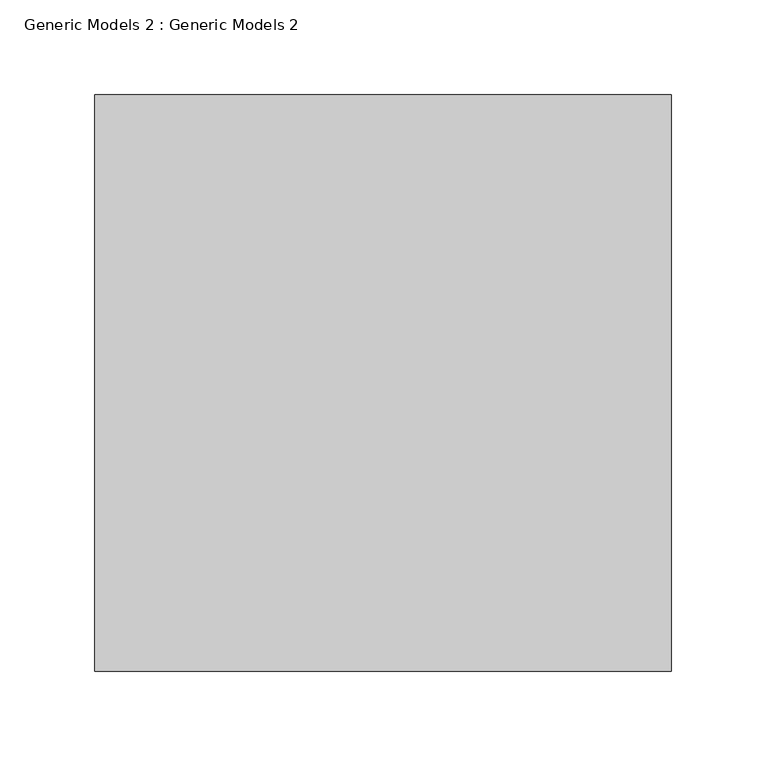
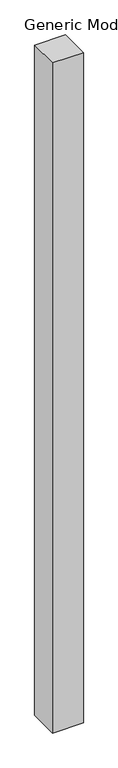
"""IFC4 building model written with IfcOpenShell, lengths in millimetres: proxy geometry, Generic Models 2 : Generic Models 2."""

from ifc_helpers import new_model, si_unit, origin, origin_with_axes, place, context, project, spatial, polyline, outline, extrude, source, transform, mapped, element, save


def generic_models_2_generic_models_2_628e6232(model_context):
    return source(origin(), model_context, "Body", "SweptSolid", [
        extrude(outline(polyline([(-8177.3519453, 3667.2444012), (-8482.1519453, 3667.2444012), (-8482.1519453, 3972.0444012), (-8177.3519453, 3972.0444012), (-8177.3519453, 3667.2444012)])), origin_with_axes(), (0.0, 0.0, 1.0), 7010.4),
    ])


if __name__ == "__main__":
    model = new_model("IFC4")
    model_context = context("Model", 3, world=origin())
    ifc_project = project(units=[si_unit("LENGTHUNIT", "METRE", prefix="MILLI")], contexts=[model_context])
    site = spatial("IfcSite", under=ifc_project)
    building = spatial("IfcBuilding", under=site)
    placement = place(None, origin())
    generic_models_2_generic_models_2_shape = generic_models_2_generic_models_2_628e6232(model_context)
    element("IfcBuildingElementProxy", 1, Name="Generic Models 2 : Generic Models 2", ObjectType="Generic Models 2 : Generic Models 2", at=placement, inside=building, context=model_context, shape_type="MappedRepresentation", body=[
        mapped(generic_models_2_generic_models_2_shape, transform((0.0, 0.0, 0.0), x_axis=(1.0, 0.0, 0.0), y_axis=(0.0, 1.0, 0.0), z_axis=(0.0, 0.0, 1.0))),
    ])
    save(model, "model.ifc")
